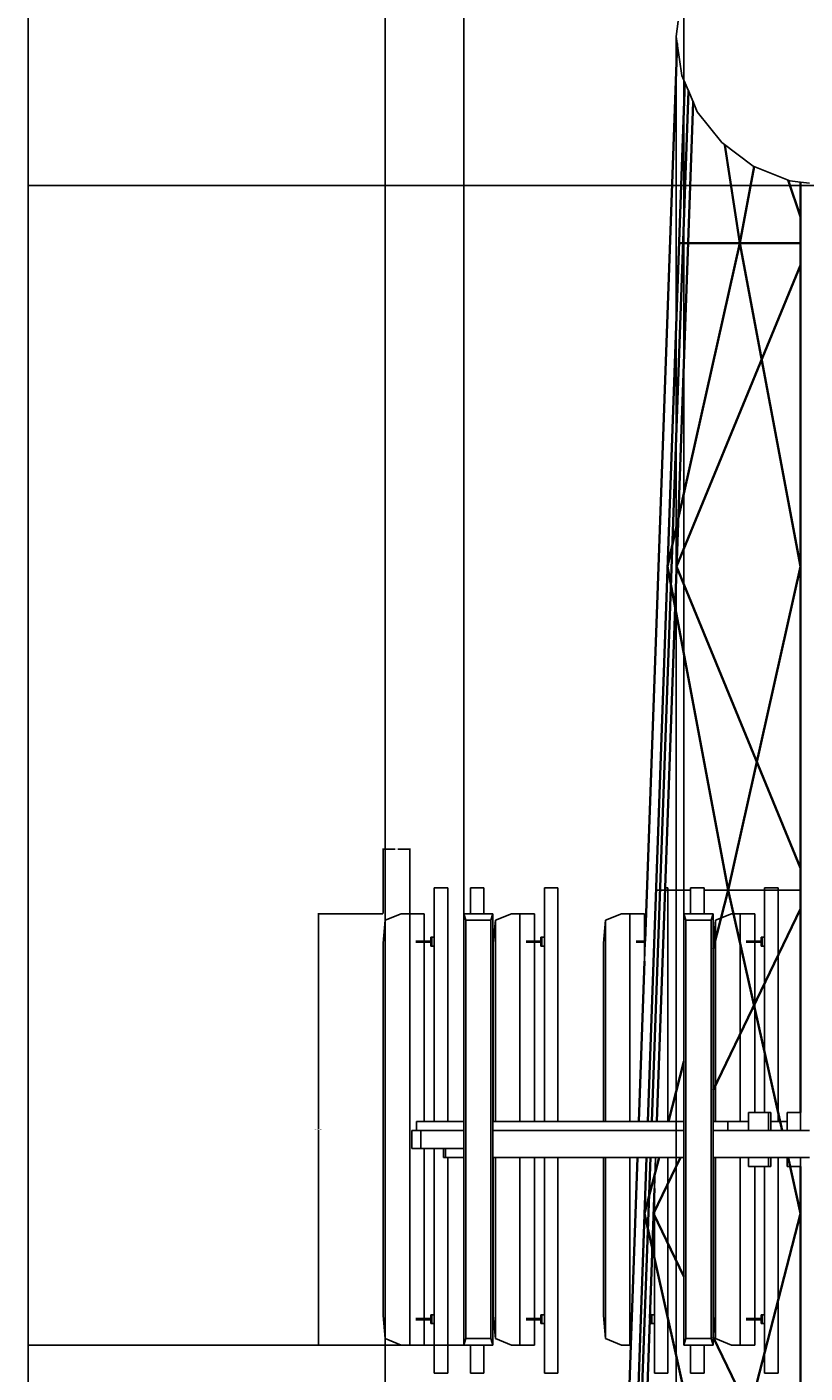
# Model space of a CAD drawing. Units: inches. Extents: x 3780 to 4301, y 1637 to 4224.
# Tile 2 of 8: x 3780 to 4040, y 3092 to 3542. Entities that reach past the tile are written whole.
import ezdxf

# ---------------------------------------------------------------- set-up
doc = ezdxf.new("R2010")
doc.units = ezdxf.units.IN
for name, color, linetype, lineweight in [('A-ANNO-DIMS', 2, 'Continuous', 18), ('E-COMM-ANTN', 4, 'Continuous', 25), ('E-COMM-DISH', 3, 'Continuous', 25), ('S-TOWR', 7, 'Continuous', 35)]:
    doc.layers.add(name, color=color, linetype=linetype, lineweight=lineweight)
doc.styles.get("Standard").update_dxf_attribs({"font": 'arial.ttf'})
doc.dimstyles.get("Standard").update_dxf_attribs({"dimtxt": 0.18, "dimasz": 0.18, "dimexe": 0.18, "dimexo": 0.0625, "dimgap": 0.09, "dimtad": 0, "dimtih": 1, "dimtoh": 1, "dimdec": 4, "dimzin": 0, "dimdsep": 46, "dimtxsty": 'Standard', "dimcen": 0.09, "dimadec": 0, "dimazin": 0, "dimtfac": 1, "dimtdec": 4, "dimtofl": 0, "dimtmove": 0, "dimatfit": 3, "dimfxl": 1, "dimtolj": 1, "dimtzin": 0, "dimarcsym": 0})

# ---------------------------------------------------------------- blocks, each defined once
blk = doc.blocks.new('ANT-PANEL')
for p, q in [((3900.05, 3833.75), (3899.34, 3826.07)), ((3905.38, 3835.91), (3900.05, 3833.75)), ((3900.05, 3694.07), (3900.05, 3833.75)), ((3905.38, 3835.91), (3908.22, 3835.91)), ((3908.22, 3691.91), (3908.22, 3835.91)), ((3899.34, 3701.75), (3899.34, 3826.07)), ((3900.05, 3694.07), (3899.34, 3701.75)), ((3905.38, 3691.91), (3900.05, 3694.07)), ((3905.38, 3691.91), (3908.22, 3691.91))]:
    blk.add_line(p, q)
blk = doc.blocks.new('ANT-PANEL-MOUNT-A')
for p, q in [((3928.47, 3835.91), (3928.47, 3844.56)), ((3928.47, 3844.56), (3932.97, 3844.56)), ((3932.97, 3835.91), (3932.97, 3844.56)), ((3926.23, 3835.91), (3926.9, 3833.75)), ((3926.23, 3835.91), (3928.47, 3835.91)), ((3926.23, 3766.56), (3926.23, 3835.91)), ((3926.9, 3694.07), (3926.9, 3833.75)), ((3926.9, 3833.75), (3935.32, 3833.75)), ((3928.47, 3835.91), (3932.97, 3835.91)), ((3932.97, 3835.91), (3935.98, 3835.91)), ((3935.98, 3835.91), (3935.32, 3833.75)), ((3935.32, 3694.07), (3935.32, 3833.75)), ((3935.98, 3766.56), (3935.98, 3835.91)), ((3936.8, 3833.75), (3936.09, 3826.07)), ((3936.8, 3766.56), (3936.8, 3833.75)), ((3936.09, 3766.56), (3936.09, 3826.07)), ((3926.23, 3763.56), (3926.23, 3766.56)), ((3936.09, 3766.56), (3935.98, 3766.56)), ((3935.98, 3763.56), (3935.98, 3766.56)), ((3936.8, 3766.56), (3936.09, 3766.56)), ((3926.23, 3757.56), (3926.23, 3763.56)), ((3935.98, 3754.56), (3935.98, 3763.56)), ((3926.23, 3754.56), (3926.23, 3757.56)), ((3926.23, 3691.91), (3926.23, 3754.56)), ((3935.98, 3691.91), (3935.98, 3754.56)), ((3935.98, 3754.56), (3936.09, 3754.56)), ((3936.09, 3701.75), (3936.09, 3754.56)), ((3936.09, 3754.56), (3936.8, 3754.56)), ((3936.8, 3694.07), (3936.8, 3754.56)), ((3936.8, 3694.07), (3936.09, 3701.75)), ((3926.23, 3691.91), (3926.9, 3694.07)), ((3926.23, 3691.91), (3928.47, 3691.91)), ((3926.9, 3694.07), (3935.32, 3694.07)), ((3928.47, 3682.56), (3928.47, 3691.91)), ((3928.47, 3691.91), (3932.97, 3691.91)), ((3932.97, 3682.56), (3932.97, 3691.91)), ((3932.97, 3691.91), (3935.98, 3691.91)), ((3935.98, 3691.91), (3935.32, 3694.07)), ((3932.97, 3682.56), (3928.47, 3682.56))]:
    blk.add_line(p, q)
blk = doc.blocks.new('*D5')
at = {"layer": 'A-ANNO-DIMS', "color": 0, "lineweight": -2, "transparency": 16777216}
for p, q in [((3899.27, 3245.56), (3877.56, 3245.56)), ((3877.74, 3245.38), (3877.74, 3173.74)), ((3877.74, 3101.74), (3877.74, 3173.38)), ((3899.27, 3101.56), (3877.56, 3101.56))]:
    blk.add_line(p, q, dxfattribs=at)
at = {"layer": 'A-ANNO-DIMS', "color": 0, "transparency": 16777216}
for points in [[(3877.71, 3245.38), (3877.77, 3245.38), (3877.74, 3245.56)], [(3877.71, 3101.74), (3877.77, 3101.74), (3877.74, 3101.56)]]:
    blk.add_solid(points, dxfattribs=at)
at = {"layer": 'Defpoints', "color": 0, "transparency": 16777216}
for p in [(3877.74, 3245.56), (3899.34, 3245.56), (3899.34, 3101.56)]:
    blk.add_point(p, dxfattribs=at)
at = {"layer": 'A-ANNO-DIMS', "color": 0, "transparency": 16777216, "insert": (3877.74, 3173.56), "char_height": 0.18, "attachment_point": 5}
blk.add_mtext('\\A1;PANEL ANTENNA 144 TYP.', dxfattribs=at)
blk = doc.blocks.new('*D6')
at = {"layer": 'A-ANNO-DIMS', "color": 0, "lineweight": -2, "transparency": 16777216}
for p, q in [((3899.34, 3245.63), (3899.34, 3267.34)), ((3899.52, 3267.16), (3903.32, 3267.16)), ((3908.04, 3267.16), (3904.24, 3267.16)), ((3908.22, 3245.63), (3908.22, 3267.34))]:
    blk.add_line(p, q, dxfattribs=at)
at = {"layer": 'A-ANNO-DIMS', "color": 0, "transparency": 16777216}
for points in [[(3899.52, 3267.19), (3899.52, 3267.13), (3899.34, 3267.16)], [(3908.04, 3267.19), (3908.04, 3267.13), (3908.22, 3267.16)]]:
    blk.add_solid(points, dxfattribs=at)
at = {"layer": 'Defpoints', "color": 0, "transparency": 16777216}
for p in [(3908.22, 3267.16), (3899.34, 3245.56), (3908.22, 3245.56)]:
    blk.add_point(p, dxfattribs=at)
at = {"layer": 'A-ANNO-DIMS', "color": 0, "transparency": 16777216, "insert": (3903.78, 3267.16), "char_height": 0.18, "attachment_point": 5}
blk.add_mtext('\\A1;9 TYP.', dxfattribs=at)
blk = doc.blocks.new('*D11')
at = {"layer": 'A-ANNO-DIMS', "color": 0, "lineweight": -2, "transparency": 16777216}
for p, q in [((3916.19, 4105.28), (3780.66, 4105.28)), ((3780.84, 4105.1), (3780.84, 2930.44)), ((3780.84, 1755.43), (3780.84, 2930.08)), ((3934.09, 1755.25), (3780.66, 1755.25))]:
    blk.add_line(p, q, dxfattribs=at)
at = {"layer": 'A-ANNO-DIMS', "color": 0, "transparency": 16777216}
for points in [[(3780.81, 4105.1), (3780.87, 4105.1), (3780.84, 4105.28)], [(3780.81, 1755.43), (3780.87, 1755.43), (3780.84, 1755.25)]]:
    blk.add_solid(points, dxfattribs=at)
at = {"layer": 'Defpoints', "color": 0, "transparency": 16777216}
for p in [(3780.84, 4105.28), (3916.25, 4105.28), (3934.15, 1755.25)]:
    blk.add_point(p, dxfattribs=at)
at = {"layer": 'A-ANNO-DIMS', "color": 0, "transparency": 16777216, "insert": (3780.84, 2930.26), "char_height": 0.18, "attachment_point": 5}
blk.add_mtext('\\A1;2350', dxfattribs=at)
blk = doc.blocks.new('*D21')
at = {"layer": 'A-ANNO-DIMS', "color": 0, "lineweight": -2, "transparency": 16777216}
for p, q in [((4010.55, 3901.46), (4300.89, 3901.46)), ((4300.71, 3901.28), (4300.71, 3685.65)), ((4300.71, 3469.64), (4300.71, 3685.28)), ((4044.72, 3469.46), (4300.89, 3469.46))]:
    blk.add_line(p, q, dxfattribs=at)
at = {"layer": 'A-ANNO-DIMS', "color": 0, "transparency": 16777216}
for points in [[(4300.68, 3901.28), (4300.74, 3901.28), (4300.71, 3901.46)], [(4300.68, 3469.64), (4300.74, 3469.64), (4300.71, 3469.46)]]:
    blk.add_solid(points, dxfattribs=at)
at = {"layer": 'Defpoints', "color": 0, "transparency": 16777216}
for p in [(4010.49, 3901.46), (4300.71, 3901.46), (4044.66, 3469.46)]:
    blk.add_point(p, dxfattribs=at)
at = {"layer": 'A-ANNO-DIMS', "color": 0, "transparency": 16777216, "insert": (4300.71, 3685.46), "char_height": 0.18, "attachment_point": 5}
blk.add_mtext('\\A1;432', dxfattribs=at)
blk = doc.blocks.new('*D22')
at = {"layer": 'A-ANNO-DIMS', "color": 0, "lineweight": -2, "transparency": 16777216}
for p, q in [((3900.05, 3694.01), (3900.05, 1636.57)), ((4181.5, 3694.01), (4181.5, 1636.57)), ((3900.23, 1636.75), (4040.31, 1636.75)), ((4181.32, 1636.75), (4041.24, 1636.75))]:
    blk.add_line(p, q, dxfattribs=at)
at = {"layer": 'A-ANNO-DIMS', "color": 0, "transparency": 16777216}
for points in [[(3900.23, 1636.78), (3900.23, 1636.72), (3900.05, 1636.75)], [(4181.32, 1636.78), (4181.32, 1636.72), (4181.5, 1636.75)]]:
    blk.add_solid(points, dxfattribs=at)
at = {"layer": 'Defpoints', "color": 0, "transparency": 16777216}
for p in [(3900.05, 3694.07), (4181.5, 3694.07), (4181.5, 1636.75)]:
    blk.add_point(p, dxfattribs=at)
at = {"layer": 'A-ANNO-DIMS', "color": 0, "transparency": 16777216, "insert": (4040.77, 1636.75), "char_height": 0.18, "attachment_point": 5}
blk.add_mtext('\\A1;281.45', dxfattribs=at)
blk = doc.blocks.new('*D26')
at = {"layer": 'A-ANNO-DIMS', "color": 0, "lineweight": -2, "transparency": 16777216}
for p, q in [((3926.17, 3101.56), (3780.66, 3101.56)), ((3780.84, 3101.38), (3780.84, 2428.59)), ((3780.84, 1755.43), (3780.84, 2428.22)), ((3934.09, 1755.25), (3780.66, 1755.25))]:
    blk.add_line(p, q, dxfattribs=at)
at = {"layer": 'A-ANNO-DIMS', "color": 0, "transparency": 16777216}
for points in [[(3780.81, 3101.38), (3780.87, 3101.38), (3780.84, 3101.56)], [(3780.81, 1755.43), (3780.87, 1755.43), (3780.84, 1755.25)]]:
    blk.add_solid(points, dxfattribs=at)
at = {"layer": 'Defpoints', "color": 0, "transparency": 16777216}
for p in [(3780.84, 3101.56), (3926.23, 3101.56), (3934.15, 1755.25)]:
    blk.add_point(p, dxfattribs=at)
at = {"layer": 'A-ANNO-DIMS', "color": 0, "transparency": 16777216, "insert": (3780.84, 2428.41), "char_height": 0.18, "attachment_point": 5}
blk.add_mtext('\\A1;1346.3', dxfattribs=at)
blk = doc.blocks.new('*D27')
at = {"layer": 'A-ANNO-DIMS', "color": 0, "lineweight": -2, "transparency": 16777216}
for p, q in [((4048.31, 3488.69), (3780.66, 3488.69)), ((3780.84, 3488.51), (3780.84, 3295.31)), ((3780.84, 3101.74), (3780.84, 3294.94)), ((3926.17, 3101.56), (3780.66, 3101.56))]:
    blk.add_line(p, q, dxfattribs=at)
at = {"layer": 'A-ANNO-DIMS', "color": 0, "transparency": 16777216}
for points in [[(3780.81, 3488.51), (3780.87, 3488.51), (3780.84, 3488.69)], [(3780.81, 3101.74), (3780.87, 3101.74), (3780.84, 3101.56)]]:
    blk.add_solid(points, dxfattribs=at)
at = {"layer": 'Defpoints', "color": 0, "transparency": 16777216}
for p in [(3780.84, 3488.69), (4048.37, 3488.69), (3926.23, 3101.56)]:
    blk.add_point(p, dxfattribs=at)
at = {"layer": 'A-ANNO-DIMS', "color": 0, "transparency": 16777216, "insert": (3780.84, 3295.13), "char_height": 0.18, "attachment_point": 5}
blk.add_mtext('\\A1;387.1', dxfattribs=at)
blk = doc.blocks.new('*D28')
at = {"layer": 'A-ANNO-DIMS', "color": 0, "lineweight": -2, "transparency": 16777216}
for p, q in [((3926.17, 3691.91), (3780.66, 3691.91)), ((3780.84, 3691.73), (3780.84, 3590.48)), ((3780.84, 3488.87), (3780.84, 3590.12)), ((4048.31, 3488.69), (3780.66, 3488.69))]:
    blk.add_line(p, q, dxfattribs=at)
at = {"layer": 'A-ANNO-DIMS', "color": 0, "transparency": 16777216}
for points in [[(3780.81, 3691.73), (3780.87, 3691.73), (3780.84, 3691.91)], [(3780.81, 3488.87), (3780.87, 3488.87), (3780.84, 3488.69)]]:
    blk.add_solid(points, dxfattribs=at)
at = {"layer": 'Defpoints', "color": 0, "transparency": 16777216}
for p in [(3780.84, 3691.91), (3926.23, 3691.91), (4048.37, 3488.69)]:
    blk.add_point(p, dxfattribs=at)
at = {"layer": 'A-ANNO-DIMS', "color": 0, "transparency": 16777216, "insert": (3780.84, 3590.3), "char_height": 0.18, "attachment_point": 5}
blk.add_mtext('\\A1;203.2', dxfattribs=at)
blk = doc.blocks.new('*D42')
at = {"layer": 'A-ANNO-DIMS', "color": 0, "lineweight": -2, "transparency": 16777216}
for p, q in [((3997.15, 3538.4), (3997.15, 1636.57)), ((4098.15, 3539.64), (4098.15, 1636.57)), ((3997.33, 1636.75), (4047.38, 1636.75)), ((4097.97, 1636.75), (4047.91, 1636.75))]:
    blk.add_line(p, q, dxfattribs=at)
at = {"layer": 'A-ANNO-DIMS', "color": 0, "transparency": 16777216}
for points in [[(3997.33, 1636.78), (3997.33, 1636.72), (3997.15, 1636.75)], [(4097.97, 1636.78), (4097.97, 1636.72), (4098.15, 1636.75)]]:
    blk.add_solid(points, dxfattribs=at)
at = {"layer": 'Defpoints', "color": 0, "transparency": 16777216}
for p in [(3997.15, 3538.47), (4098.15, 3539.7), (4098.15, 1636.75)]:
    blk.add_point(p, dxfattribs=at)
at = {"layer": 'A-ANNO-DIMS', "color": 0, "transparency": 16777216, "insert": (4047.65, 1636.75), "char_height": 0.18, "attachment_point": 5}
blk.add_mtext('\\A1;101', dxfattribs=at)
blk = doc.blocks.new('*D45')
at = {"layer": 'A-ANNO-DIMS', "color": 0, "lineweight": -2, "transparency": 16777216}
for p, q in [((3971.79, 3552.9), (3780.66, 3552.9)), ((3780.84, 3552.72), (3780.84, 3520.98)), ((3780.84, 3488.87), (3780.84, 3520.61)), ((4048.31, 3488.69), (3780.66, 3488.69))]:
    blk.add_line(p, q, dxfattribs=at)
at = {"layer": 'A-ANNO-DIMS', "color": 0, "transparency": 16777216}
for points in [[(3780.81, 3552.72), (3780.87, 3552.72), (3780.84, 3552.9)], [(3780.81, 3488.87), (3780.87, 3488.87), (3780.84, 3488.69)]]:
    blk.add_solid(points, dxfattribs=at)
at = {"layer": 'Defpoints', "color": 0, "transparency": 16777216}
for p in [(3780.84, 3552.9), (3971.85, 3552.9), (4048.37, 3488.69)]:
    blk.add_point(p, dxfattribs=at)
at = {"layer": 'A-ANNO-DIMS', "color": 0, "transparency": 16777216, "insert": (3780.84, 3520.8), "char_height": 0.18, "attachment_point": 5}
blk.add_mtext('\\A1;64.21', dxfattribs=at)
blk = doc.blocks.new('*D48')
at = {"layer": 'A-ANNO-DIMS', "color": 0, "lineweight": -2, "transparency": 16777216}
for p, q in [((3926.23, 3245.63), (3926.23, 4223.96)), ((3926.41, 4223.78), (3962.66, 4223.78)), ((3999.55, 4223.78), (3963.31, 4223.78)), ((3999.73, 3245.63), (3999.73, 4223.96))]:
    blk.add_line(p, q, dxfattribs=at)
at = {"layer": 'A-ANNO-DIMS', "color": 0, "transparency": 16777216}
for points in [[(3926.41, 4223.81), (3926.41, 4223.75), (3926.23, 4223.78)], [(3999.55, 4223.81), (3999.55, 4223.75), (3999.73, 4223.78)]]:
    blk.add_solid(points, dxfattribs=at)
at = {"layer": 'Defpoints', "color": 0, "transparency": 16777216}
for p in [(3999.73, 4223.78), (3926.23, 3245.56), (3999.73, 3245.56)]:
    blk.add_point(p, dxfattribs=at)
at = {"layer": 'A-ANNO-DIMS', "color": 0, "transparency": 16777216, "insert": (3962.98, 4223.78), "char_height": 0.18, "attachment_point": 5}
blk.add_mtext('\\A1;73.5', dxfattribs=at)
blk = doc.blocks.new('*D49')
at = {"layer": 'A-ANNO-DIMS', "color": 0, "lineweight": -2, "transparency": 16777216}
for p, q in [((3999.73, 3245.63), (3999.73, 4223.96)), ((3999.91, 4223.78), (4036.16, 4223.78)), ((4073.05, 4223.78), (4036.81, 4223.78)), ((4073.23, 3245.63), (4073.23, 4223.96))]:
    blk.add_line(p, q, dxfattribs=at)
at = {"layer": 'A-ANNO-DIMS', "color": 0, "transparency": 16777216}
for points in [[(3999.91, 4223.81), (3999.91, 4223.75), (3999.73, 4223.78)], [(4073.05, 4223.81), (4073.05, 4223.75), (4073.23, 4223.78)]]:
    blk.add_solid(points, dxfattribs=at)
at = {"layer": 'Defpoints', "color": 0, "transparency": 16777216}
for p in [(4073.23, 4223.78), (3999.73, 3245.56), (4073.23, 3245.56)]:
    blk.add_point(p, dxfattribs=at)
at = {"layer": 'A-ANNO-DIMS', "color": 0, "transparency": 16777216, "insert": (4036.48, 4223.78), "char_height": 0.18, "attachment_point": 5}
blk.add_mtext('\\A1;73.5', dxfattribs=at)

msp = doc.modelspace()

# ---------------------------------------------------------------- linework, layer by layer
at = {"layer": 'E-COMM-ANTN'}
for p, q in [((3916.394, 3237.7144), (3916.394, 3254.2144)), ((3920.894, 3254.2144), (3916.394, 3254.2144)), ((3920.894, 3176.2144), (3920.894, 3254.2144)), ((3953.144, 3237.7144), (3953.144, 3254.2144)), ((3953.144, 3254.2144), (3957.644, 3254.2144)), ((3957.644, 3176.2144), (3957.644, 3254.2144)), ((3993.465, 3254.2144), (3994.394, 3254.2144)), ((3994.394, 3176.2144), (3994.394, 3254.2144)), ((4001.9676, 3245.5639), (4001.9676, 3254.2144)), ((4006.4676, 3254.2144), (4001.9676, 3254.2144)), ((4006.4676, 3245.5639), (4006.4676, 3254.2144)), ((4026.644, 3237.7144), (4026.644, 3254.2144)), ((4026.644, 3254.2144), (4031.144, 3254.2144)), ((4031.144, 3176.2144), (4031.144, 3254.2144)), ((3990.4384, 3253.4644), (4001.9676, 3253.4644)), ((4001.9676, 3253.4644), (3993.4384, 3253.4644)), ((4006.4676, 3253.4644), (4014.5503, 3253.4644)), ((4038.6622, 3253.4644), (4006.4676, 3253.4644)), ((4014.5503, 3253.4644), (4038.6622, 3253.4644)), ((3913.0928, 3245.5639), (3908.2178, 3245.5639)), ((3913.0928, 3236.4019), (3913.0928, 3245.5639)), ((3942.1336, 3245.5639), (3936.7982, 3243.4039)), ((3942.1336, 3245.5639), (3944.9678, 3245.5639)), ((3944.9678, 3176.2144), (3944.9678, 3245.5639)), ((3949.8428, 3245.5639), (3944.9678, 3245.5639)), ((3949.8428, 3236.4019), (3949.8428, 3245.5639)), ((3978.8836, 3245.5639), (3973.5482, 3243.4039)), ((3978.8836, 3245.5639), (3981.7178, 3245.5639)), ((3981.7178, 3176.2144), (3981.7178, 3245.5639)), ((3986.5928, 3245.5639), (3981.7178, 3245.5639)), ((3986.5928, 3236.4019), (3986.5928, 3245.5639)), ((3999.7315, 3245.5639), (4000.3979, 3243.4039)), ((3999.7315, 3245.5639), (4001.9676, 3245.5639)), ((3999.7315, 3176.2144), (3999.7315, 3245.5639)), ((4001.9676, 3245.5639), (4006.4676, 3245.5639)), ((4006.4676, 3245.5639), (4009.4815, 3245.5639)), ((4009.4815, 3245.5639), (4008.8151, 3243.4039)), ((4009.4815, 3176.2144), (4009.4815, 3245.5639)), ((4015.6336, 3245.5639), (4010.2982, 3243.4039)), ((4015.6336, 3245.5639), (4018.4678, 3245.5639)), ((4018.4678, 3176.2144), (4018.4678, 3245.5639)), ((4023.3428, 3245.5639), (4018.4678, 3245.5639)), ((4023.3428, 3236.4019), (4023.3428, 3245.5639)), ((3973.5482, 3243.4039), (3972.8371, 3235.7215)), ((3973.5482, 3176.2144), (3973.5482, 3243.4039)), ((4000.3979, 3103.7239), (4000.3979, 3243.4039)), ((4000.3979, 3243.4039), (4008.8151, 3243.4039)), ((4008.8151, 3103.7239), (4008.8151, 3243.4039)), ((4010.2982, 3243.4039), (4009.5871, 3235.7215)), ((4010.2982, 3176.2144), (4010.2982, 3243.4039)), ((3910.2873, 3236.4019), (3913.0928, 3236.4019)), ((3910.2873, 3236.0269), (3913.0928, 3236.0269)), ((3915.2457, 3236.4019), (3913.0928, 3236.4019)), ((3913.0928, 3176.2144), (3913.0928, 3236.0269)), ((3913.0928, 3236.0269), (3915.2457, 3236.0269)), ((3915.2457, 3237.7144), (3915.5705, 3237.7144)), ((3915.2457, 3237.7144), (3915.2457, 3236.4019)), ((3915.2457, 3236.4019), (3915.2457, 3236.0269)), ((3915.2457, 3236.0269), (3915.2457, 3234.7144)), ((3915.5705, 3234.7144), (3915.5705, 3237.7144)), ((3915.5705, 3237.7144), (3916.394, 3237.7144)), ((3916.394, 3234.7144), (3916.394, 3237.7144)), ((3947.0373, 3236.4019), (3949.8428, 3236.4019)), ((3947.0373, 3236.0269), (3949.8428, 3236.0269)), ((3951.9957, 3236.4019), (3949.8428, 3236.4019)), ((3949.8428, 3176.2144), (3949.8428, 3236.0269)), ((3949.8428, 3236.0269), (3951.9957, 3236.0269)), ((3951.9957, 3237.7144), (3952.3205, 3237.7144)), ((3951.9957, 3237.7144), (3951.9957, 3236.4019)), ((3951.9957, 3236.4019), (3951.9957, 3236.0269)), ((3951.9957, 3236.0269), (3951.9957, 3234.7144)), ((3952.3205, 3237.7144), (3953.144, 3237.7144)), ((3952.3205, 3234.7144), (3952.3205, 3237.7144)), ((3953.144, 3234.7144), (3953.144, 3237.7144)), ((3983.7873, 3236.4019), (3986.5928, 3236.4019)), ((3983.7873, 3236.0269), (3986.5928, 3236.0269)), ((3986.8315, 3236.4019), (3986.5928, 3236.4019)), ((3986.5928, 3229.691), (3986.5928, 3236.0269)), ((3986.5928, 3236.0269), (3986.8182, 3236.0269)), ((3986.5928, 3229.691), (3986.8182, 3236.0269)), ((3986.8182, 3236.0269), (3986.8315, 3236.4019)), ((4020.5373, 3236.4019), (4023.3428, 3236.4019)), ((4020.5373, 3236.0269), (4023.3428, 3236.0269)), ((4025.4957, 3236.4019), (4023.3428, 3236.4019)), ((4023.3428, 3179.2144), (4023.3428, 3236.0269)), ((4023.3428, 3236.0269), (4025.4957, 3236.0269)), ((4025.4957, 3237.7144), (4025.8205, 3237.7144)), ((4025.4957, 3237.7144), (4025.4957, 3236.4019)), ((4025.4957, 3236.4019), (4025.4957, 3236.0269)), ((4025.4957, 3236.0269), (4025.4957, 3234.7144)), ((4025.8205, 3237.7144), (4026.644, 3237.7144)), ((4025.8205, 3234.7144), (4025.8205, 3237.7144)), ((4026.644, 3234.7144), (4026.644, 3237.7144)), ((3915.2457, 3234.7144), (3915.5705, 3234.7144)), ((3915.5705, 3234.7144), (3916.394, 3234.7144)), ((3916.394, 3176.2144), (3916.394, 3234.7144)), ((3951.9957, 3234.7144), (3952.3205, 3234.7144)), ((3952.3205, 3234.7144), (3953.144, 3234.7144)), ((3953.144, 3176.2144), (3953.144, 3234.7144)), ((3972.8371, 3176.2144), (3972.8371, 3235.7215)), ((4009.5871, 3176.2144), (4009.5871, 3235.7215)), ((4025.4957, 3234.7144), (4025.8205, 3234.7144)), ((4025.8205, 3234.7144), (4026.644, 3234.7144)), ((4026.644, 3179.2144), (4026.644, 3234.7144)), ((4021.2379, 3179.2144), (4023.3428, 3179.2144)), ((4021.2379, 3176.2144), (4021.2379, 3179.2144)), ((4023.3428, 3179.2144), (4026.644, 3179.2144)), ((4026.644, 3179.2144), (4027.9879, 3179.2144)), ((4027.9879, 3179.2144), (4027.9879, 3173.2144)), ((4027.9879, 3179.2144), (4028.7541, 3179.2144)), ((4028.7541, 3179.2144), (4028.7541, 3176.2144)), ((4038.6622, 3179.2144), (4034.2176, 3179.2144)), ((4034.2176, 3179.2144), (4034.2176, 3176.2144)), ((4038.6622, 3173.2144), (4038.6622, 3179.2144)), ((3908.976, 3167.2144), (3908.976, 3173.2144)), ((3908.976, 3173.2144), (3910.4676, 3173.2144)), ((3910.4676, 3173.2144), (3910.4676, 3176.2144)), ((3910.4676, 3176.2144), (3913.0928, 3176.2144)), ((3910.4676, 3173.2144), (3911.9591, 3173.2144)), ((3911.9591, 3173.2144), (3911.9591, 3167.2144)), ((3926.2315, 3173.2144), (3911.9591, 3173.2144)), ((3913.0928, 3176.2144), (3916.394, 3176.2144)), ((3916.394, 3176.2144), (3920.894, 3176.2144)), ((3920.894, 3176.2144), (3926.2315, 3176.2144)), ((3999.7315, 3173.2144), (3935.9815, 3173.2144)), ((3936.7982, 3176.2144), (3944.9678, 3176.2144)), ((3944.9678, 3176.2144), (3949.8428, 3176.2144)), ((3949.8428, 3176.2144), (3953.144, 3176.2144)), ((3953.144, 3176.2144), (3957.644, 3176.2144)), ((3972.8371, 3176.2144), (3957.644, 3176.2144)), ((3973.5482, 3176.2144), (3972.8371, 3176.2144)), ((3981.7178, 3176.2144), (3973.5482, 3176.2144)), ((3984.6909, 3176.2144), (3981.7178, 3176.2144)), ((3987.6909, 3176.2144), (3984.6909, 3176.2144)), ((3988.9899, 3176.2144), (3987.6909, 3176.2144)), ((3990.6909, 3176.2144), (3988.9899, 3176.2144)), ((3994.394, 3176.2144), (3990.6909, 3176.2144)), ((3999.7315, 3176.2144), (3994.394, 3176.2144)), ((3999.7315, 3173.2144), (3999.7315, 3176.2144)), ((3999.7315, 3164.2144), (3999.7315, 3173.2144)), ((4009.4815, 3176.2144), (4009.5871, 3176.2144)), ((4009.4815, 3173.2144), (4009.4815, 3176.2144)), ((4014.3906, 3173.2144), (4009.4815, 3173.2144)), ((4009.4815, 3164.2144), (4009.4815, 3173.2144)), ((4009.5871, 3176.2144), (4010.2982, 3176.2144)), ((4010.2982, 3176.2144), (4014.3906, 3176.2144)), ((4014.3906, 3173.2144), (4014.3906, 3176.2144)), ((4014.3906, 3176.2144), (4018.4678, 3176.2144)), ((4021.2379, 3173.2144), (4014.3906, 3173.2144)), ((4018.4678, 3176.2144), (4021.2379, 3176.2144)), ((4021.2379, 3173.2144), (4021.2379, 3176.2144)), ((4027.9879, 3173.2144), (4021.2379, 3173.2144)), ((4028.7541, 3173.2144), (4027.9879, 3173.2144)), ((4028.7541, 3176.2144), (4028.7541, 3173.2144)), ((4031.144, 3176.2144), (4028.7541, 3176.2144)), ((4034.2176, 3173.2144), (4028.7541, 3173.2144)), ((4034.2176, 3176.2144), (4031.144, 3176.2144)), ((4034.2176, 3176.2144), (4034.2176, 3173.2144)), ((4038.6622, 3173.2144), (4034.2176, 3173.2144)), ((4041.6622, 3173.2144), (4038.6622, 3173.2144)), ((3911.9591, 3167.2144), (3908.976, 3167.2144)), ((3911.9591, 3167.2144), (3913.0928, 3167.2144)), ((3913.0928, 3110.4019), (3913.0928, 3167.2144)), ((3913.0928, 3167.2144), (3916.394, 3167.2144)), ((3916.394, 3111.7144), (3916.394, 3167.2144)), ((3916.394, 3167.2144), (3919.4676, 3167.2144)), ((3919.4676, 3164.2144), (3919.4676, 3167.2144)), ((3919.4676, 3167.2144), (3920.1171, 3167.2144)), ((3920.1171, 3164.2144), (3919.4676, 3164.2144)), ((3920.1171, 3164.2144), (3920.1171, 3167.2144)), ((3920.1171, 3167.2144), (3926.2315, 3167.2144)), ((3920.894, 3164.2144), (3920.1171, 3164.2144)), ((3920.894, 3092.2144), (3920.894, 3164.2144)), ((3926.2315, 3164.2144), (3920.894, 3164.2144)), ((3936.7982, 3164.2144), (3944.9678, 3164.2144)), ((3944.9678, 3101.5639), (3944.9678, 3164.2144)), ((3944.9678, 3164.2144), (3949.8428, 3164.2144)), ((3949.8428, 3110.4019), (3949.8428, 3164.2144)), ((3949.8428, 3164.2144), (3953.144, 3164.2144)), ((3953.144, 3111.7144), (3953.144, 3164.2144)), ((3953.144, 3164.2144), (3957.644, 3164.2144)), ((3957.644, 3092.2144), (3957.644, 3164.2144)), ((3957.644, 3164.2144), (3972.8371, 3164.2144)), ((3972.8371, 3111.4063), (3972.8371, 3164.2144)), ((3972.8371, 3164.2144), (3973.5482, 3164.2144)), ((3973.5482, 3103.7239), (3973.5482, 3164.2144)), ((3973.5482, 3164.2144), (3981.7178, 3164.2144)), ((3981.7178, 3101.5639), (3981.7178, 3164.2144)), ((3981.7178, 3164.2144), (3984.2641, 3164.2144)), ((3984.2641, 3164.2144), (3987.2641, 3164.2144)), ((3987.2641, 3164.2144), (3988.5631, 3164.2144)), ((3988.5631, 3164.2144), (3990.2641, 3164.2144)), ((3989.894, 3153.8097), (3990.2641, 3164.2144)), ((3990.2641, 3164.2144), (3994.394, 3164.2144)), ((3994.394, 3092.2144), (3994.394, 3164.2144)), ((3994.394, 3164.2144), (3999.7315, 3164.2144)), ((3999.7315, 3101.5639), (3999.7315, 3164.2144)), ((4009.4815, 3164.2144), (4009.5871, 3164.2144)), ((4009.4815, 3101.5639), (4009.4815, 3164.2144)), ((4009.5871, 3111.4063), (4009.5871, 3164.2144)), ((4009.5871, 3164.2144), (4010.2982, 3164.2144)), ((4010.2982, 3103.7239), (4010.2982, 3164.2144)), ((4010.2982, 3164.2144), (4018.4678, 3164.2144)), ((4018.4678, 3101.5639), (4018.4678, 3164.2144)), ((4018.4678, 3164.2144), (4021.2379, 3164.2144)), ((4021.2379, 3161.2144), (4021.2379, 3164.2144)), ((4021.2379, 3164.2144), (4027.9879, 3164.2144)), ((4027.9879, 3164.2144), (4027.9879, 3161.2144)), ((4027.9879, 3164.2144), (4028.7541, 3164.2144)), ((4028.7541, 3164.2144), (4028.7541, 3161.2144)), ((4028.7541, 3164.2144), (4031.144, 3164.2144)), ((4031.144, 3092.2144), (4031.144, 3164.2144)), ((4034.2176, 3164.2144), (4031.144, 3164.2144)), ((4034.2176, 3164.2144), (4034.2176, 3161.2144)), ((4034.2176, 3164.2144), (4038.6622, 3164.2144)), ((4038.6622, 3161.2144), (4038.6622, 3164.2144)), ((4038.6622, 3164.2144), (4041.6622, 3164.2144)), ((4021.2379, 3161.2144), (4023.3428, 3161.2144)), ((4023.3428, 3110.4019), (4023.3428, 3161.2144)), ((4026.644, 3161.2144), (4023.3428, 3161.2144)), ((4026.644, 3111.7144), (4026.644, 3161.2144)), ((4027.9879, 3161.2144), (4026.644, 3161.2144)), ((4027.9879, 3161.2144), (4028.7541, 3161.2144)), ((4034.2176, 3161.2144), (4038.6622, 3161.2144)), ((3989.894, 3111.7144), (3989.894, 3153.8097)), ((3910.2873, 3110.4019), (3913.0928, 3110.4019)), ((3915.2457, 3110.4019), (3913.0928, 3110.4019)), ((3915.2457, 3111.7144), (3915.5705, 3111.7144)), ((3915.2457, 3111.7144), (3915.2457, 3110.4019)), ((3915.2457, 3110.4019), (3915.2457, 3110.0269)), ((3915.5705, 3108.7144), (3915.5705, 3111.7144)), ((3915.5705, 3111.7144), (3916.394, 3111.7144)), ((3916.394, 3108.7144), (3916.394, 3111.7144)), ((3947.0373, 3110.4019), (3949.8428, 3110.4019)), ((3951.9957, 3110.4019), (3949.8428, 3110.4019)), ((3951.9957, 3111.7144), (3952.3205, 3111.7144)), ((3951.9957, 3111.7144), (3951.9957, 3110.4019)), ((3951.9957, 3110.4019), (3951.9957, 3110.0269)), ((3952.3205, 3108.7144), (3952.3205, 3111.7144)), ((3952.3205, 3111.7144), (3953.144, 3111.7144)), ((3953.144, 3108.7144), (3953.144, 3111.7144)), ((3973.5482, 3103.7239), (3972.8371, 3111.4063)), ((3988.3368, 3110.0269), (3988.3502, 3110.4019)), ((3988.3502, 3110.4019), (3988.7457, 3110.4019)), ((3988.7457, 3111.7144), (3989.0705, 3111.7144)), ((3988.7457, 3111.7144), (3988.7457, 3110.4019)), ((3988.7457, 3110.4019), (3988.7457, 3110.0269)), ((3989.0705, 3108.7144), (3989.0705, 3111.7144)), ((3989.0705, 3111.7144), (3989.894, 3111.7144)), ((3989.894, 3108.7144), (3989.894, 3111.7144)), ((4010.2982, 3103.7239), (4009.5871, 3111.4063)), ((4020.5373, 3110.4019), (4023.3428, 3110.4019)), ((4025.4957, 3110.4019), (4023.3428, 3110.4019)), ((4025.4957, 3111.7144), (4025.8205, 3111.7144)), ((4025.4957, 3111.7144), (4025.4957, 3110.4019)), ((4025.4957, 3110.4019), (4025.4957, 3110.0269)), ((4025.8205, 3108.7144), (4025.8205, 3111.7144)), ((4025.8205, 3111.7144), (4026.644, 3111.7144)), ((4026.644, 3108.7144), (4026.644, 3111.7144)), ((3910.2873, 3110.0269), (3913.0928, 3110.0269)), ((3913.0928, 3101.5639), (3913.0928, 3110.0269)), ((3913.0928, 3110.0269), (3915.2457, 3110.0269)), ((3915.2457, 3110.0269), (3915.2457, 3108.7144)), ((3915.2457, 3108.7144), (3915.5705, 3108.7144)), ((3915.5705, 3108.7144), (3916.394, 3108.7144)), ((3916.394, 3092.2144), (3916.394, 3108.7144)), ((3947.0373, 3110.0269), (3949.8428, 3110.0269)), ((3949.8428, 3101.5639), (3949.8428, 3110.0269)), ((3949.8428, 3110.0269), (3951.9957, 3110.0269)), ((3951.9957, 3110.0269), (3951.9957, 3108.7144)), ((3951.9957, 3108.7144), (3952.3205, 3108.7144)), ((3952.3205, 3108.7144), (3953.144, 3108.7144)), ((3953.144, 3092.2144), (3953.144, 3108.7144)), ((3988.3368, 3110.0269), (3988.7457, 3110.0269)), ((3988.7457, 3110.0269), (3988.7457, 3108.7144)), ((3988.7457, 3108.7144), (3989.0705, 3108.7144)), ((3989.0705, 3108.7144), (3989.894, 3108.7144)), ((3989.894, 3092.2144), (3989.894, 3108.7144)), ((4020.5373, 3110.0269), (4023.3428, 3110.0269)), ((4023.3428, 3101.5639), (4023.3428, 3110.0269)), ((4023.3428, 3110.0269), (4025.4957, 3110.0269)), ((4025.4957, 3110.0269), (4025.4957, 3108.7144)), ((4025.4957, 3108.7144), (4025.8205, 3108.7144)), ((4025.8205, 3108.7144), (4026.644, 3108.7144)), ((4026.644, 3092.2144), (4026.644, 3108.7144)), ((3913.0928, 3101.5639), (3908.2178, 3101.5639)), ((3942.1336, 3101.5639), (3936.7982, 3103.7239)), ((3942.1336, 3101.5639), (3944.9678, 3101.5639)), ((3949.8428, 3101.5639), (3944.9678, 3101.5639)), ((3978.8836, 3101.5639), (3973.5482, 3103.7239)), ((3978.8836, 3101.5639), (3981.7178, 3101.5639)), ((3982.0358, 3101.5639), (3981.7178, 3101.5639)), ((3999.7315, 3101.5639), (4000.3979, 3103.7239)), ((3999.7315, 3101.5639), (4001.9676, 3101.5639)), ((4000.3979, 3103.7239), (4008.8151, 3103.7239)), ((4001.9676, 3092.2144), (4001.9676, 3101.5639)), ((4001.9676, 3101.5639), (4006.4676, 3101.5639)), ((4006.4676, 3092.2144), (4006.4676, 3101.5639)), ((4006.4676, 3101.5639), (4009.4815, 3101.5639)), ((4009.4815, 3101.5639), (4008.8151, 3103.7239)), ((4015.6336, 3101.5639), (4010.2982, 3103.7239)), ((4015.6336, 3101.5639), (4018.4678, 3101.5639)), ((4023.3428, 3101.5639), (4018.4678, 3101.5639)), ((3916.394, 3092.2144), (3920.894, 3092.2144)), ((3953.144, 3092.2144), (3957.644, 3092.2144)), ((3989.894, 3092.2144), (3994.394, 3092.2144)), ((4001.9676, 3092.2144), (4006.4676, 3092.2144)), ((4026.644, 3092.2144), (4031.144, 3092.2144))]:
    msp.add_line(p, q, dxfattribs=at)
at = {"layer": 'E-COMM-DISH'}
for p, q in [((3997.7575, 3543.6033), (3997.1451, 3538.4672)), ((3997.1451, 3538.4672), (3997.4898, 3536.0752)), ((3997.4898, 3536.0752), (3999.0215, 3525.4453)), ((3999.0215, 3525.4453), (4000.0282, 3523.0965)), ((4000.0282, 3523.0965), (4001.2277, 3520.2977)), ((4001.2277, 3520.2977), (4002.7983, 3516.633)), ((4002.7983, 3516.633), (4004.2042, 3513.3527)), ((4004.2042, 3513.3527), (4012.3399, 3503.0137)), ((4012.3399, 3503.0137), (4022.8743, 3495.1326)), ((4022.8743, 3495.1326), (4035.0894, 3490.2468)), ((4035.0894, 3490.2468), (4038.6622, 3489.8207)), ((4038.6622, 3489.8207), (4041.6622, 3489.463))]:
    msp.add_line(p, q, dxfattribs=at)
at = {"layer": 'S-TOWR'}
for p, q in [((3986.8315, 3236.4019), (3997.4898, 3536.0752)), ((4000.0282, 3523.0965), (3987.6909, 3176.2144)), ((3988.9899, 3176.2144), (4001.2277, 3520.2977)), ((4002.7983, 3516.633), (3993.465, 3254.2144)), ((4013.4094, 3502.2135), (4018.3914, 3469.4644)), ((4018.3914, 3469.4644), (4023.1858, 3495.008)), ((4034.523, 3490.4733), (4038.6622, 3478.2927)), ((4038.6622, 3489.8207), (4038.6622, 3179.2144)), ((4018.3914, 3469.4644), (3994.2795, 3361.4644)), ((3998.1207, 3469.4644), (4018.3914, 3469.4644)), ((4038.6622, 3469.4644), (4001.1207, 3469.4644)), ((4038.6622, 3361.4644), (4018.3914, 3469.4644)), ((4038.6622, 3462.1643), (3997.2795, 3361.4644)), ((3994.2795, 3361.4644), (4014.5503, 3253.4644)), ((3997.2795, 3361.4644), (4038.6622, 3260.7646)), ((4014.5503, 3253.4644), (4038.6622, 3361.4644)), ((3990.6909, 3176.2144), (3993.465, 3254.2144)), ((4014.5503, 3253.4644), (4009.4815, 3233.8805)), ((4032.4668, 3173.2144), (4014.5503, 3253.4644)), ((4038.6622, 3247.2414), (4009.4815, 3186.711)), ((3984.6909, 3176.2144), (3986.5928, 3229.691)), ((3999.7315, 3196.2102), (3994.5561, 3176.2144)), ((3987.2641, 3164.2144), (3937.1525, 1755.2487)), ((3938.4515, 1755.2487), (3988.5631, 3164.2144)), ((3982.0358, 3101.5639), (3984.2641, 3164.2144)), ((3991.4502, 3164.2144), (3986.5972, 3145.4644)), ((3998.6363, 3164.2144), (3989.5972, 3145.4644)), ((4038.6622, 3145.4644), (4034.4761, 3164.2144)), ((4038.6622, 1755.2487), (4038.6622, 3161.2144)), ((3989.894, 3153.8097), (3988.3502, 3110.4019)), ((3986.5972, 3145.4644), (4010.7091, 3037.4644)), ((3989.5972, 3145.4644), (3999.7315, 3124.4426)), ((4010.7091, 3037.4644), (4038.6622, 3145.4644)), ((3988.3368, 3110.0269), (3940.1525, 1755.2487)), ((3934.1525, 1755.2487), (3982.0358, 3101.5639)), ((4009.4815, 3104.2179), (4038.6622, 3043.6874))]:
    msp.add_line(p, q, dxfattribs=at)

# ---------------------------------------------------------------- block references
at = {"layer": 'E-COMM-ANTN'}
for name in ['ANT-PANEL-MOUNT-A', 'ANT-PANEL']:
    msp.add_blockref(name, (0, -590.3438), dxfattribs=at)

# ---------------------------------------------------------------- dimensions: what is measured, and where the dimension line sits
at = {"layer": 'A-ANNO-DIMS'}
for base, p1, p2, override, picture, middle in [((3999.7315, 4223.7769), (3926.2315, 3245.5639), (3999.7315, 3245.5639), {"dimdec": 1, "dimlfac": 1, "dimrnd": 0, "dimzin": 0, "dimdsep": 46, "dimlunit": 2}, '*D48', (3962.9815, 4223.7769)), ((4073.2315, 4223.7769), (3999.7315, 3245.5639), (4073.2315, 3245.5639), {"dimdec": 1, "dimlfac": 1, "dimrnd": 0, "dimzin": 0, "dimdsep": 46, "dimlunit": 2}, '*D49', (4036.4815, 4223.7769)), ((4181.498, 1636.7487), (3900.0482, 3694.0677), (4181.498, 3694.0677), {"dimdec": 2, "dimlfac": 1, "dimrnd": 0, "dimzin": 0, "dimdsep": 46, "dimlunit": 2}, '*D22', (4040.7731, 1636.7487)), ((4098.1498, 1636.7487), (3997.1451, 3538.4672), (4098.1498, 3539.6986), {"dimdec": 0, "dimlfac": 1, "dimrnd": 0, "dimzin": 0, "dimdsep": 46, "dimlunit": 2}, '*D42', (4047.6474, 1636.7487))]:
    dim = msp.add_linear_dim(base=base, p1=p1, p2=p2, dimstyle='Standard', override=override, dxfattribs=at)
    dim.commit()
    dim.dimension.update_dxf_attribs({"geometry": picture, "text_midpoint": middle})
for base, p1, p2, override, picture, middle in [((3780.8371, 4105.2769), (3934.1525, 1755.2487), (3916.252, 4105.2769), {"dimdec": 0, "dimlfac": 1, "dimrnd": 0, "dimzin": 0, "dimdsep": 46, "dimlunit": 2}, '*D11', (3780.8371, 2930.2628)), ((4300.7091, 3901.4644), (4044.6622, 3469.4644), (4010.4853, 3901.4644), {"dimdec": 0, "dimlfac": 1, "dimrnd": 0, "dimzin": 0, "dimdsep": 46, "dimlunit": 2}, '*D21', (4300.7091, 3685.4644)), ((3780.8371, 3691.9077), (4048.3735, 3488.689), (3926.2315, 3691.9077), {"dimdec": 1, "dimlfac": 1, "dimrnd": 0, "dimzin": 0, "dimdsep": 46, "dimlunit": 2}, '*D28', (3780.8371, 3590.2983)), ((3780.8371, 3552.903), (4048.3735, 3488.689), (3971.8516, 3552.903), {"dimdec": 2, "dimlfac": 1, "dimrnd": 0, "dimzin": 0, "dimdsep": 46, "dimlunit": 2}, '*D45', (3780.8371, 3520.796)), ((3780.8371, 3488.689), (3926.2315, 3101.5639), (4048.3735, 3488.689), {"dimdec": 1, "dimlfac": 1, "dimrnd": 0, "dimzin": 0, "dimdsep": 46, "dimlunit": 2}, '*D27', (3780.8371, 3295.1265)), ((3780.8371, 3101.5639), (3934.1525, 1755.2487), (3926.2315, 3101.5639), {"dimdec": 1, "dimlfac": 1, "dimrnd": 0, "dimzin": 0, "dimdsep": 46, "dimlunit": 2}, '*D26', (3780.8371, 2428.4063))]:
    dim = msp.add_linear_dim(base=base, p1=p1, p2=p2, angle=90, dimstyle='Standard', override=override, dxfattribs=at)
    dim.commit()
    dim.dimension.update_dxf_attribs({"geometry": picture, "text_midpoint": middle})
dim = msp.add_linear_dim(base=(3908.2178, 3267.1639), p1=(3899.3371, 3245.5639), p2=(3908.2178, 3245.5639), text='<> TYP.', dimstyle='Standard', override={"dimdec": 0, "dimlfac": 1, "dimrnd": 0, "dimzin": 0, "dimdsep": 46, "dimlunit": 2}, dxfattribs=at)
dim.commit()
dim.dimension.update_dxf_attribs({"geometry": '*D6', "text_midpoint": (3903.7775, 3267.1639)})
dim = msp.add_linear_dim(base=(3877.7371, 3245.5639), p1=(3899.3371, 3101.5639), p2=(3899.3371, 3245.5639), angle=90, text='PANEL ANTENNA <> TYP.', dimstyle='Standard', override={"dimdec": 0, "dimlfac": 1, "dimrnd": 0, "dimzin": 0, "dimdsep": 46, "dimlunit": 2}, dxfattribs=at)
dim.commit()
dim.dimension.update_dxf_attribs({"geometry": '*D5', "text_midpoint": (3877.7371, 3173.5639)})

doc.saveas('drawing.dxf')
